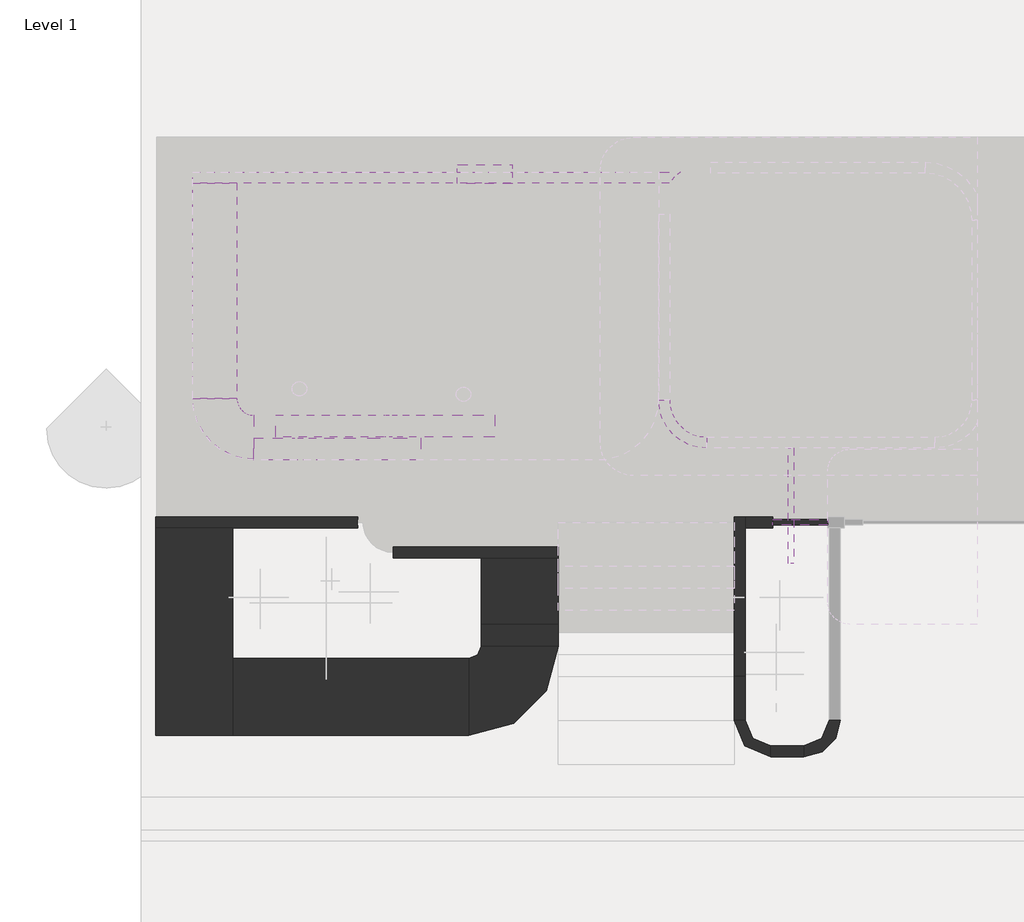
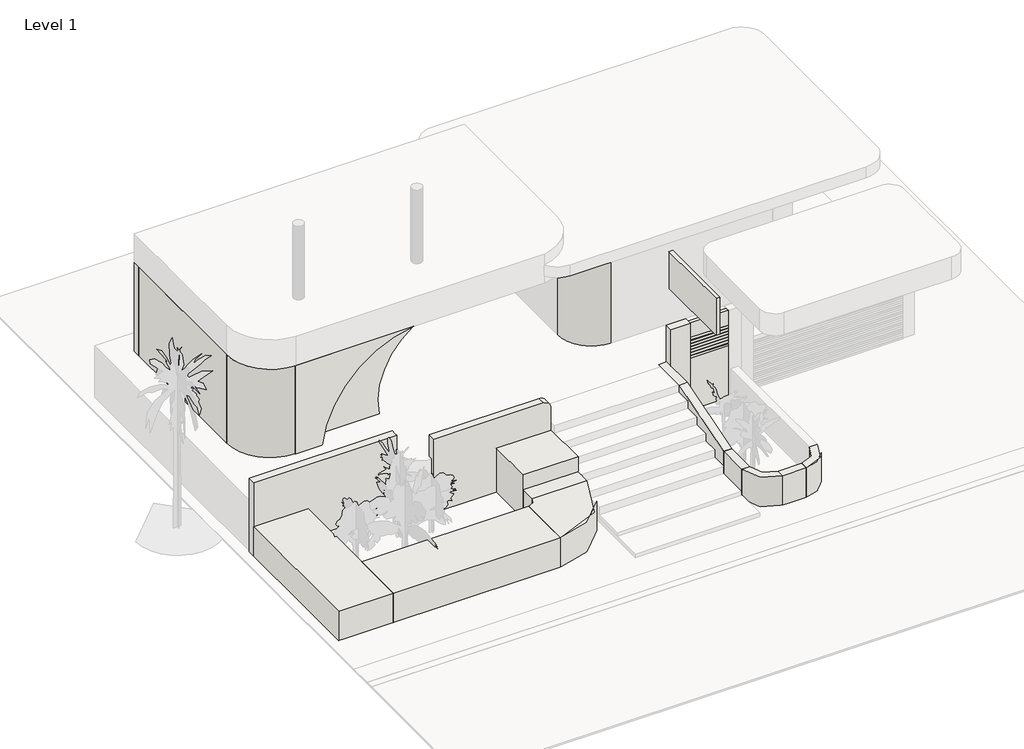
# One storey, part 1 of 2: 23 walls, 1 window.
"""IFC4 building model written with IfcOpenShell, lengths in millimetres."""

from ifc_helpers import new_model, si_unit, point, frame, frame_2d, origin, origin_with_axes, place, context, project, spatial, polyline, circle_curve, trimmed, segment, composite_curve, outline, extrude, faceted_brep, transform, mapped, element, save
from ifc_brep_helpers import plane_surface, cylinder_surface, revolved_surface, advanced_brep
from components import window_e9f06afb

model = new_model("IFC4")

# Units and contexts
model_context = context("Model", 3, world=origin())
ifc_project = project(units=[si_unit("LENGTHUNIT", "METRE", prefix="MILLI")], contexts=[model_context])

# Site, building, storey
site = spatial("IfcSite", under=ifc_project)
building = spatial("IfcBuilding", under=site)
storey = spatial("IfcBuildingStorey", under=building, Name="Level 1", Elevation=0.0)

# Walls
placement = place(None, origin())
element("IfcWall", 1, ObjectType="Generic - 12\" white", at=placement, inside=storey, context=model_context, shape_type="SweptSolid", body=[
    extrude(outline(composite_curve([segment(polyline([(0.0, -6972.7035766), (2743.2, -6972.7035766)]), True, "CONTINUOUS"), segment(trimmed(circle_curve(frame_2d((2743.2, -7277.5035766)), 304.8), [point((2743.2, -6972.7035766))], [point((3048.0, -7277.5035766))], False, "CARTESIAN"), True, "CONTINUOUS"), segment(polyline([(3048.0, -7277.5035766), (3048.0, -11546.5074836), (0.0, -11546.5074836), (0.0, -6972.7035766)]), True, "CONTINUOUS")], self_intersect=False)), frame((0.0, 4157.34911, 0.0), z_axis=(0.0, 1.0, 0.0), x_axis=(0.0, 0.0, 1.0)), (0.0, 0.0, 1.0), 304.8),
])
element("IfcWall", 2, ObjectType="Generic - 12\" white", at=placement, inside=storey, context=model_context, shape_type="AdvancedBrep", body=[
    advanced_brep(
    [(-12522.0257411, 5297.0999244, 0.0), (-18123.3035766, 5297.0999244, 0.0), (-18123.3035766, 5297.0999244, 3048.0), (-12522.0257411, 5297.0999244, 3048.0), (-12522.0257411, 4992.2999244, 0.0), (-12522.0257411, 4992.2999244, 3048.0), (-18123.3035766, 4992.2999244, 3048.0), (-18123.3035766, 4992.2999244, 1219.2), (-18123.3035766, 4992.2999244, 0.0), (-15989.7035766, 4992.2999244, 0.0)],
    [
        (0, 1),
        (1, 2),
        (2, 3),
        (3, 0),
        (4, 5),
        (5, 6),
        (6, 7),
        (7, 8),
        (8, 9),
        (9, 4),
        (0, 4, circle_curve(frame((-11546.5074836, 5144.6999244, 0.0), z_axis=(0.0, 0.0, 1.0), x_axis=(1.0, 0.0, 0.0)), 987.3508144)),
        (8, 1),
        (2, 6),
        (5, 3, circle_curve(frame((-11546.5074836, 5144.6999244, 3048.0), z_axis=(0.0, 0.0, -1.0), x_axis=(1.0, 0.0, 0.0)), 987.3508144)),
    ],
    [
        plane_surface(frame((-11670.258298, 5297.0999244, 0.0), z_axis=(0.0, 1.0, 0.0), x_axis=(-1.0, 0.0, 0.0))),
        plane_surface(frame((-11670.258298, 4992.2999244, 0.0), z_axis=(0.0, -1.0, 0.0), x_axis=(1.0, 0.0, 0.0))),
        plane_surface(frame((-12381.458298, 5297.0999244, 0.0), z_axis=(0.0, 0.0, -1.0), x_axis=(0.0, -1.0, 0.0))),
        plane_surface(frame((-17056.5035766, 5297.0999244, 3048.0), z_axis=(0.0, 0.0, 1.0), x_axis=(0.0, -1.0, 0.0))),
        revolved_surface(polyline([(-10559.1566692, 5144.6999244, 3048.0), (-10559.1566692, 5144.6999244, 0.0)]), (-11546.5074836, 5144.6999244, 0.0), (0.0, 0.0, 1.0)),
        plane_surface(frame((-18123.3035766, 4992.2999244, 0.0), z_axis=(-1.0, 0.0, 0.0), x_axis=(0.0, -1.0, 0.0))),
    ],
    [
        (0, [[1, 2, 3, 4]]),
        (1, [[5, 6, 7, 8, 9, 10]]),
        (2, [[-1, 11, -10, -9, 12]]),
        (3, [[-3, 13, -6, 14]]),
        (4, [[-4, -14, -5, -11]]),
        (5, [[-2, -12, -8, -7, -13]]),
    ],
),
])
element("IfcWall", 3, ObjectType="Generic - 12\" white", at=placement, inside=storey, context=model_context, shape_type="Brep", body=[
    faceted_brep([(-2095.9035766, 5297.0999244, 0.0), (-2095.9035766, 877.4999244, 0.0), (-2095.9035766, 877.4999244, 1219.2), (-2095.9035766, 3900.0999244, 2133.6), (-2095.9035766, 5297.0999244, 2133.6), (-1791.1035766, 5297.0999244, 0.0), (-1791.1035766, 5297.0999244, 2133.6), (-1791.1035766, 3900.0999244, 2133.6), (-1791.1035766, 877.4999244, 1219.2), (-1791.1035766, 877.4999244, 0.0), (-1791.1035766, 4992.2999244, 0.0)], [[[0, 1, 2, 3, 4]], [[5, 6, 7, 8, 9, 10]], [[1, 0, 5, 10, 9]], [[2, 1, 9, 8]], [[4, 3, 7, 6]], [[3, 2, 8, 7]], [[0, 4, 6, 5]]]),
])
element("IfcWall", 4, ObjectType="Generic - 12\" white", at=placement, inside=storey, context=model_context, shape_type="SweptSolid", body=[
    extrude(outline(polyline([(-2095.9035766, -341.7000756), (-2095.9035766, 877.4999244), (-1791.1035766, 877.4999244), (-1791.1035766, -341.7000756), (-2095.9035766, -341.7000756)])), origin_with_axes(), (0.0, 0.0, 1.0), 1219.2),
])
element("IfcWall", 5, ObjectType="Generic - 12\" white", at=placement, inside=storey, context=model_context, shape_type="SweptSolid", body=[
    extrude(outline(composite_curve([segment(polyline([(-1081.398989, -1051.4046632), (-1081.398989, -1356.2046632)]), True, "CONTINUOUS"), segment(trimmed(circle_curve(frame_2d((-1081.398989, -341.7000756)), 1014.5045876), [point((-1081.398989, -1356.2046632))], [point((-2095.9035766, -341.7000756))], False, "CARTESIAN"), True, "CONTINUOUS"), segment(polyline([(-2095.9035766, -341.7000756), (-1791.1035766, -341.7000756)]), True, "CONTINUOUS"), segment(trimmed(circle_curve(frame_2d((-1081.398989, -341.7000756)), 709.7045876), [point((-1791.1035766, -341.7000756))], [point((-1081.398989, -1051.4046632))], True, "CARTESIAN"), True, "CONTINUOUS")], self_intersect=False)), origin_with_axes(), (0.0, 0.0, 1.0), 1219.2),
])
element("IfcWall", 6, ObjectType="Generic - 12\" white", at=placement, inside=storey, context=model_context, shape_type="SweptSolid", body=[
    extrude(outline(polyline([(-166.998989, -1356.2046632), (-1081.398989, -1356.2046632), (-1081.398989, -1051.4046632), (-166.998989, -1051.4046632), (-166.998989, -1356.2046632)])), origin_with_axes(), (0.0, 0.0, 1.0), 1219.2),
])
element("IfcWall", 7, ObjectType="Generic - 12\" white", at=placement, inside=storey, context=model_context, shape_type="SweptSolid", body=[
    extrude(outline(composite_curve([segment(polyline([(542.7055987, -341.7000756), (847.5055987, -341.7000756)]), True, "CONTINUOUS"), segment(trimmed(circle_curve(frame_2d((-166.998989, -341.7000756)), 1014.5045876), [point((847.5055987, -341.7000756))], [point((-166.998989, -1356.2046632))], False, "CARTESIAN"), True, "CONTINUOUS"), segment(polyline([(-166.998989, -1356.2046632), (-166.998989, -1051.4046632)]), True, "CONTINUOUS"), segment(trimmed(circle_curve(frame_2d((-166.998989, -341.7000756)), 709.7045876), [point((-166.998989, -1051.4046632))], [point((542.7055987, -341.7000756))], True, "CARTESIAN"), True, "CONTINUOUS")], self_intersect=False)), origin_with_axes(), (0.0, 0.0, 1.0), 1219.2),
])
element("IfcWall", 8, ObjectType="Generic - 12\" white", at=placement, inside=storey, context=model_context, shape_type="Brep", body=[
    faceted_brep([(-1791.1035766, 4992.2999244, 0.0), (-1029.1035766, 4992.2999244, 0.0), (-1029.1035766, 4992.2999244, 3657.6), (-1791.1035766, 4992.2999244, 3657.6), (-1791.1035766, 5297.0999244, 0.0), (-1791.1035766, 5297.0999244, 2133.6), (-1791.1035766, 5297.0999244, 3657.6), (-1029.1035766, 5297.0999244, 3657.6), (-1029.1035766, 5297.0999244, 0.0), (-1029.1035766, 5220.8999244, 0.0), (-1029.1035766, 5068.4999244, 0.0)], [[[0, 1, 2, 3]], [[4, 5, 6, 7, 8]], [[1, 0, 4, 8, 9, 10]], [[3, 2, 7, 6]], [[0, 3, 6, 5, 4]], [[1, 10, 9, 8, 7, 2]]]),
])
element("IfcWall", 9, ObjectType="Generic - 12\" white", at=placement, inside=storey, context=model_context, shape_type="AdvancedBrep", body=[
    advanced_brep(
    [(-2854.0500691, 7504.6568058, 6096.0), (-3887.0438771, 8537.6506138, 6096.0), (-4191.8438771, 8537.6506138, 6096.0), (-2854.0500691, 7199.8568058, 6096.0), (-2854.0500691, 7504.6568058, 2133.6), (-2854.0500691, 7199.8568058, 2133.6), (-4191.8438771, 8537.6506138, 2133.6), (-3887.0438771, 8537.6506138, 2133.6), (-3887.0438771, 8537.6506138, 5791.2), (-4191.8438771, 8537.6506138, 5791.2)],
    [
        (0, 1, circle_curve(frame((-2854.0500691, 8537.6506138, 6096.0), z_axis=(0.0, 0.0, -1.0), x_axis=(1.0, 0.0, 0.0)), 1032.993808)),
        (1, 2),
        (2, 3, circle_curve(frame((-2854.0500691, 8537.6506138, 6096.0), z_axis=(0.0, 0.0, 1.0), x_axis=(1.0, 0.0, 0.0)), 1337.793808)),
        (3, 0),
        (4, 5),
        (5, 6, circle_curve(frame((-2854.0500691, 8537.6506138, 2133.6), z_axis=(0.0, 0.0, -1.0), x_axis=(1.0, 0.0, 0.0)), 1337.793808)),
        (6, 7),
        (7, 4, circle_curve(frame((-2854.0500691, 8537.6506138, 2133.6), z_axis=(0.0, 0.0, 1.0), x_axis=(1.0, 0.0, 0.0)), 1032.993808)),
        (0, 4),
        (7, 8),
        (8, 1),
        (6, 9),
        (9, 2),
        (5, 3),
    ],
    [
        plane_surface(frame((-1821.0562611, 8537.6506138, 6096.0), z_axis=(0.0, 0.0, 1.0), x_axis=(0.0, -1.0, 0.0))),
        plane_surface(frame((-1821.0562611, 8537.6506138, 2133.6), z_axis=(0.0, 0.0, -1.0), x_axis=(0.0, 1.0, 0.0))),
        revolved_surface(polyline([(-1821.0562611000003, 8537.6506138, 2133.6), (-1821.0562611000003, 8537.6506138, 6096.0)]), (-2854.0500691, 8537.6506138, 2133.6), (0.0, 0.0, -1.0)),
        plane_surface(frame((-3887.0438771, 8537.6506138, 6096.0), z_axis=(0.0, 1.0, 0.0), x_axis=(0.0, 0.0, -1.0))),
        cylinder_surface(frame((-2854.0500691, 8537.6506138, 2133.6), z_axis=(0.0, 0.0, 1.0), x_axis=(1.0, 0.0, 0.0)), 1337.793808),
        plane_surface(frame((-2854.0500691, 7199.8568058, 6096.0), z_axis=(1.0, 0.0, 0.0), x_axis=(0.0, 0.0, -1.0))),
    ],
    [
        (0, [[1, 2, 3, 4]]),
        (1, [[5, 6, 7, 8]]),
        (2, [[-1, 9, -8, 10, 11]]),
        (3, [[-2, -11, -10, -7, 12, 13]]),
        (4, [[-3, -13, -12, -6, 14]]),
        (5, [[-4, -14, -5, -9]]),
    ],
),
])
element("IfcWall", 10, ObjectType="Generic - 12\" white", at=placement, inside=storey, context=model_context, shape_type="AdvancedBrep", body=[
    advanced_brep(
    [(-3588.9235033, 14853.6629979, 2133.6), (-17097.1000691, 14853.6629979, 2133.6), (-17097.1000691, 14853.6629979, 5791.2), (-3588.9235033, 14853.6629979, 5791.2), (-5792.0438771, 14853.6629979, 2193.4133489), (-4191.8438771, 14853.6629979, 2193.4133489), (-4191.8438771, 14853.6629979, 5393.8133489), (-5792.0438771, 14853.6629979, 5393.8133489), (-9774.0964397, 14853.6629979, 2997.2), (-6738.7964397, 14853.6629979, 2997.2), (-6738.7964397, 14853.6629979, 5435.6), (-9774.0964397, 14853.6629979, 5435.6), (-17097.1000691, 14548.8629979, 2133.6), (-15877.9000691, 14548.8629979, 2133.6), (-3900.9068004, 14548.8629979, 2133.6), (-3900.9068004, 14548.8629979, 5791.2), (-15877.9000691, 14548.8629979, 5791.2), (-17097.1000691, 14548.8629979, 5791.2), (-4191.8438771, 14548.8629979, 2193.4133489), (-5792.0438771, 14548.8629979, 2193.4133489), (-5792.0438771, 14548.8629979, 5393.8133489), (-4191.8438771, 14548.8629979, 5393.8133489), (-9774.0964397, 14548.8629979, 5435.6), (-6738.7964397, 14548.8629979, 5435.6), (-6738.7964397, 14548.8629979, 2997.2), (-9774.0964397, 14548.8629979, 2997.2)],
    [
        (0, 1),
        (1, 2),
        (2, 3),
        (3, 0),
        (4, 5),
        (5, 6),
        (6, 7),
        (7, 4),
        (8, 9),
        (9, 10),
        (10, 11),
        (11, 8),
        (12, 13),
        (13, 14),
        (14, 15),
        (15, 16),
        (16, 17),
        (17, 12),
        (18, 19),
        (19, 20),
        (20, 21),
        (21, 18),
        (22, 23),
        (23, 24),
        (24, 25),
        (25, 22),
        (3, 15, circle_curve(frame((-2746.2869957, 13679.0999244, 5791.2), z_axis=(0.0, 0.0, 1.0), x_axis=(1.0, 0.0, 0.0)), 1445.5568814)),
        (14, 0, circle_curve(frame((-2746.2869957, 13679.0999244, 2133.6), z_axis=(0.0, 0.0, -1.0), x_axis=(1.0, 0.0, 0.0)), 1445.5568814)),
        (12, 1),
        (2, 17),
        (4, 19),
        (18, 5),
        (21, 6),
        (20, 7),
        (24, 9),
        (8, 25),
        (23, 10),
        (22, 11),
    ],
    [
        plane_surface(frame((-3538.3964397, 14853.6629979, 2133.6), z_axis=(0.0, 1.0, 0.0), x_axis=(-1.0, 0.0, 0.0))),
        plane_surface(frame((-3538.3964397, 14548.8629979, 2133.6), z_axis=(0.0, -1.0, 0.0), x_axis=(1.0, 0.0, 0.0))),
        revolved_surface(polyline([(-1300.7301142999997, 13679.0999244, 5791.2), (-1300.7301142999997, 13679.0999244, 2133.6)]), (-2746.2869957, 13679.0999244, 2133.6), (0.0, 0.0, 1.0)),
        plane_surface(frame((-3538.3964397, 14853.6629979, 2133.6), z_axis=(0.0, 0.0, -1.0), x_axis=(0.0, -1.0, 0.0))),
        plane_surface(frame((-16487.5000691, 14853.6629979, 5791.2), z_axis=(0.0, 0.0, 1.0), x_axis=(0.0, -1.0, 0.0))),
        plane_surface(frame((-5792.0438771, 14853.6629979, 2193.4133489), z_axis=(0.0, 0.0, 1.0), x_axis=(0.0, -1.0, 0.0))),
        plane_surface(frame((-4191.8438771, 14853.6629979, 2193.4133489), z_axis=(-1.0, 0.0, 0.0), x_axis=(0.0, -1.0, 0.0))),
        plane_surface(frame((-4191.8438771, 14853.6629979, 5393.8133489), z_axis=(0.0, 0.0, -1.0), x_axis=(0.0, -1.0, 0.0))),
        plane_surface(frame((-5792.0438771, 14853.6629979, 5393.8133489), z_axis=(1.0, 0.0, 0.0), x_axis=(0.0, -1.0, 0.0))),
        plane_surface(frame((-8262.7964397, 13329.6629979, 2997.2), z_axis=(0.0, 0.0, 1.0), x_axis=(0.0, 1.0, 0.0))),
        plane_surface(frame((-6738.7964397, 13329.6629979, 2997.2), z_axis=(-1.0, 0.0, 0.0), x_axis=(0.0, 1.0, 0.0))),
        plane_surface(frame((-6738.7964397, 13329.6629979, 5435.6), z_axis=(0.0, 0.0, -1.0), x_axis=(0.0, 1.0, 0.0))),
        plane_surface(frame((-9774.0964397, 13329.6629979, 5435.6), z_axis=(1.0, 0.0, 0.0), x_axis=(0.0, 1.0, 0.0))),
        plane_surface(frame((-17097.1000691, 14701.2629979, 2133.6), z_axis=(-1.0, 0.0, 0.0), x_axis=(0.0, -1.0, 0.0))),
    ],
    [
        (0, [[1, 2, 3, 4], [5, 6, 7, 8], [9, 10, 11, 12]]),
        (1, [[13, 14, 15, 16, 17, 18], [19, 20, 21, 22], [23, 24, 25, 26]]),
        (2, [[-4, 27, -15, 28]]),
        (3, [[-1, -28, -14, -13, 29]]),
        (4, [[-3, 30, -17, -16, -27]]),
        (5, [[-5, 31, -19, 32]]),
        (6, [[-6, -32, -22, 33]]),
        (7, [[-7, -33, -21, 34]]),
        (8, [[-8, -34, -20, -31]]),
        (9, [[35, -9, 36, -25]]),
        (10, [[37, -10, -35, -24]]),
        (11, [[-37, -23, 38, -11]]),
        (12, [[-38, -26, -36, -12]]),
        (13, [[-2, -29, -18, -30]]),
    ],
),
])
element("IfcWall", 11, ObjectType="Generic - 2'", at=placement, inside=storey, context=model_context, shape_type="AdvancedBrep", body=[
    advanced_brep(
    [(-14800.2693346, 7502.2322633, 5791.2), (-14800.2693346, 7502.2322633, 2133.6), (-11752.2693346, 7502.2322633, 2133.6), (-8736.0193346, 7502.2322633, 5791.2), (-14800.2693346, 8111.8322633, 5791.2), (-8736.0193346, 8111.8322633, 5791.2), (-11752.2693346, 8111.8322633, 2133.6), (-14800.2693346, 8111.8322633, 2133.6)],
    [
        (0, 1),
        (1, 2),
        (2, 3, circle_curve(frame((-8736.0193346, 7502.2322633, 2718.7205295), z_axis=(0.0, 1.0, 0.0), x_axis=(-1.0, 0.0, 0.0)), 3072.4794705)),
        (3, 0),
        (4, 5),
        (5, 6, circle_curve(frame((-8736.0193346, 8111.8322633, 2718.7205295), z_axis=(0.0, -1.0, 0.0), x_axis=(-1.0, 0.0, 0.0)), 3072.4794705)),
        (6, 7),
        (7, 4),
        (1, 7),
        (6, 2),
        (3, 5),
        (4, 0),
    ],
    [
        plane_surface(frame((-14800.2693346, 7502.2322633, 5791.2), z_axis=(0.0, -1.0, 0.0), x_axis=(0.0, 0.0, -1.0))),
        plane_surface(frame((-14800.2693346, 8111.8322633, 5791.2), z_axis=(0.0, 1.0, 0.0), x_axis=(0.0, 0.0, 1.0))),
        plane_surface(frame((-14800.2693346, 7502.2322633, 2133.6), z_axis=(0.0, 0.0, -1.0), x_axis=(0.0, 1.0, 0.0))),
        plane_surface(frame((-8736.0193346, 7502.2322633, 5791.2), z_axis=(0.0, 0.0, 1.0), x_axis=(0.0, 1.0, 0.0))),
        plane_surface(frame((-14800.2693346, 7502.2322633, 5791.2), z_axis=(-1.0, 0.0, 0.0), x_axis=(0.0, 1.0, 0.0))),
        revolved_surface(polyline([(-11808.4988051, 8111.8322633, 2718.7205295), (-11808.4988051, 7502.2322633, 2718.7205295)]), (-8736.0193346, 8111.8322633, 2718.7205295), (0.0, 1.0, 0.0)),
    ],
    [
        (0, [[1, 2, 3, 4]]),
        (1, [[5, 6, 7, 8]]),
        (2, [[-2, 9, -7, 10]]),
        (3, [[-4, 11, -5, 12]]),
        (4, [[-1, -12, -8, -9]]),
        (5, [[-3, -10, -6, -11]]),
    ],
),
])
element("IfcWall", 12, ObjectType="Generic - 2'", at=placement, inside=storey, context=model_context, shape_type="AdvancedBrep", body=[
    advanced_brep(
    [(-15409.8693346, 6873.8139644, 2133.6), (-14343.0693346, 6873.8139644, 2133.6), (-10776.892063, 6873.8139644, 5791.2), (-15409.8693346, 6873.8139644, 5791.2), (-15409.8693346, 7483.4139644, 2133.6), (-15409.8693346, 7483.4139644, 5791.2), (-10776.892063, 7483.4139644, 5791.2), (-14343.0693346, 7483.4139644, 2133.6), (-15409.8693346, 6892.6322633, 2133.6), (-15409.8693346, 6892.6322633, 5791.2)],
    [
        (0, 1),
        (1, 2, circle_curve(frame((-10246.3978198, 6873.8139644, 1706.6457679), z_axis=(0.0, 1.0, 0.0), x_axis=(-1.0, 0.0, 0.0)), 4118.8599657)),
        (2, 3),
        (3, 0),
        (4, 5),
        (5, 6),
        (6, 7, circle_curve(frame((-10246.3978198, 7483.4139644, 1706.6457679), z_axis=(0.0, -1.0, 0.0), x_axis=(-1.0, 0.0, 0.0)), 4118.8599657)),
        (7, 4),
        (0, 8),
        (8, 4),
        (7, 1),
        (2, 6),
        (5, 9),
        (9, 3),
    ],
    [
        plane_surface(frame((-15409.8693346, 6873.8139644, 2133.6), z_axis=(0.0, -1.0, 0.0), x_axis=(1.0, 0.0, 0.0))),
        plane_surface(frame((-15409.8693346, 7483.4139644, 2133.6), z_axis=(0.0, 1.0, 0.0), x_axis=(-1.0, 0.0, 0.0))),
        plane_surface(frame((-15409.8693346, 6873.8139644, 2133.6), z_axis=(0.0, 0.0, -1.0), x_axis=(0.0, 1.0, 0.0))),
        plane_surface(frame((-10776.892063, 6873.8139644, 5791.2), z_axis=(0.0, 0.0, 1.0), x_axis=(0.0, 1.0, 0.0))),
        plane_surface(frame((-15409.8693346, 6873.8139644, 5791.2), z_axis=(-1.0, 0.0, 0.0), x_axis=(0.0, 1.0, 0.0))),
        revolved_surface(polyline([(-14365.257785500002, 7483.4139644, 1706.6457679), (-14365.257785500002, 6873.8139644, 1706.6457679)]), (-10246.3978198, 7483.4139644, 1706.6457679), (0.0, 1.0, 0.0)),
    ],
    [
        (0, [[1, 2, 3, 4]]),
        (1, [[5, 6, 7, 8]]),
        (2, [[-1, 9, 10, -8, 11]]),
        (3, [[-3, 12, -6, 13, 14]]),
        (4, [[-4, -14, -13, -5, -10, -9]]),
        (5, [[-2, -11, -7, -12]]),
    ],
),
])
element("IfcWall", 13, ObjectType="Generic - 4' white", at=placement, inside=storey, context=model_context, shape_type="SweptSolid", body=[
    extrude(outline(polyline([(-17097.1000691, 8579.8629979), (-17097.1000691, 14548.8629979), (-15877.9000691, 14548.8629979), (-15877.9000691, 8579.8629979), (-17097.1000691, 8579.8629979)])), frame((0.0, 0.0, 2133.6), z_axis=(0.0, 0.0, 1.0), x_axis=(1.0, 0.0, 0.0)), (0.0, 0.0, 1.0), 3657.6),
])
element("IfcWall", 14, ObjectType="Generic - 4' white", at=placement, inside=storey, context=model_context, shape_type="AdvancedBrep", body=[
    advanced_brep(
    [(-15409.8693346, 8111.8322633, 5791.2), (-15877.9000691, 8579.8629979, 5791.2), (-17097.1000691, 8579.8629979, 5791.2), (-15409.8693346, 6892.6322633, 5791.2), (-15409.8693346, 7483.4139644, 5791.2), (-15409.8693346, 8111.8322633, 2133.6), (-15409.8693346, 7483.4139644, 2133.6), (-15409.8693346, 6892.6322633, 2133.6), (-17097.1000691, 8579.8629979, 2133.6), (-15877.9000691, 8579.8629979, 2133.6)],
    [
        (0, 1, circle_curve(frame((-15409.8693346, 8579.8629979, 5791.2), z_axis=(0.0, 0.0, -1.0), x_axis=(1.0, 0.0, 0.0)), 468.0307345)),
        (1, 2),
        (2, 3, circle_curve(frame((-15409.8693346, 8579.8629979, 5791.2), z_axis=(0.0, 0.0, 1.0), x_axis=(1.0, 0.0, 0.0)), 1687.2307345)),
        (3, 4),
        (4, 0),
        (5, 6),
        (6, 7),
        (7, 8, circle_curve(frame((-15409.8693346, 8579.8629979, 2133.6), z_axis=(0.0, 0.0, -1.0), x_axis=(1.0, 0.0, 0.0)), 1687.2307345)),
        (8, 9),
        (9, 5, circle_curve(frame((-15409.8693346, 8579.8629979, 2133.6), z_axis=(0.0, 0.0, 1.0), x_axis=(1.0, 0.0, 0.0)), 468.0307345)),
        (0, 5),
        (9, 1),
        (8, 2),
        (7, 3),
    ],
    [
        plane_surface(frame((-14941.8386001, 8579.8629979, 5791.2), z_axis=(0.0, 0.0, 1.0), x_axis=(0.0, -1.0, 0.0))),
        plane_surface(frame((-14941.8386001, 8579.8629979, 2133.6), z_axis=(0.0, 0.0, -1.0), x_axis=(0.0, 1.0, 0.0))),
        revolved_surface(polyline([(-14941.8386001, 8579.8629979, 2133.6), (-14941.8386001, 8579.8629979, 5791.2)]), (-15409.8693346, 8579.8629979, 2133.6), (0.0, 0.0, -1.0)),
        plane_surface(frame((-15877.9000691, 8579.8629979, 5791.2), z_axis=(0.0, 1.0, 0.0), x_axis=(0.0, 0.0, -1.0))),
        cylinder_surface(frame((-15409.8693346, 8579.8629979, 2133.6), z_axis=(0.0, 0.0, 1.0), x_axis=(1.0, 0.0, 0.0)), 1687.2307345),
        plane_surface(frame((-15409.8693346, 6892.6322633, 5791.2), z_axis=(1.0, 0.0, 0.0), x_axis=(0.0, 0.0, -1.0))),
    ],
    [
        (0, [[1, 2, 3, 4, 5]]),
        (1, [[6, 7, 8, 9, 10]]),
        (2, [[-1, 11, -10, 12]]),
        (3, [[-2, -12, -9, 13]]),
        (4, [[-3, -13, -8, 14]]),
        (5, [[-5, -4, -14, -7, -6, -11]]),
    ],
),
])
element("IfcWall", 15, ObjectType="Generic - 6\" brown", at=placement, inside=storey, context=model_context, shape_type="SweptSolid", body=[
    extrude(outline(polyline([(494.8964234, 5068.4999244), (-1029.1035766, 5068.4999244), (-1029.1035766, 5220.8999244), (494.8964234, 5220.8999244), (494.8964234, 5068.4999244)])), frame((0.0, 0.0, 2133.6), z_axis=(0.0, 0.0, 1.0), x_axis=(1.0, 0.0, 0.0)), (0.0, 0.0, 1.0), 101.6),
    extrude(outline(polyline([(494.8964234, 5068.4999244), (-1029.1035766, 5068.4999244), (-1029.1035766, 5220.8999244), (494.8964234, 5220.8999244), (494.8964234, 5068.4999244)])), frame((0.0, 0.0, 2260.6), z_axis=(0.0, 0.0, 1.0), x_axis=(1.0, 0.0, 0.0)), (0.0, 0.0, 1.0), 101.6),
    extrude(outline(polyline([(494.8964234, 5068.4999244), (-1029.1035766, 5068.4999244), (-1029.1035766, 5220.8999244), (494.8964234, 5220.8999244), (494.8964234, 5068.4999244)])), frame((0.0, 0.0, 2387.6), z_axis=(0.0, 0.0, 1.0), x_axis=(1.0, 0.0, 0.0)), (0.0, 0.0, 1.0), 101.6),
    extrude(outline(polyline([(494.8964234, 5068.4999244), (-1029.1035766, 5068.4999244), (-1029.1035766, 5220.8999244), (494.8964234, 5220.8999244), (494.8964234, 5068.4999244)])), frame((0.0, 0.0, 2514.6), z_axis=(0.0, 0.0, 1.0), x_axis=(1.0, 0.0, 0.0)), (0.0, 0.0, 1.0), 101.6),
    extrude(outline(polyline([(494.8964234, 5068.4999244), (-1029.1035766, 5068.4999244), (-1029.1035766, 5220.8999244), (494.8964234, 5220.8999244), (494.8964234, 5068.4999244)])), frame((0.0, 0.0, 2641.6), z_axis=(0.0, 0.0, 1.0), x_axis=(1.0, 0.0, 0.0)), (0.0, 0.0, 1.0), 101.6),
    extrude(outline(polyline([(494.8964234, 5068.4999244), (-1029.1035766, 5068.4999244), (-1029.1035766, 5220.8999244), (494.8964234, 5220.8999244), (494.8964234, 5068.4999244)])), frame((0.0, 0.0, 2768.6), z_axis=(0.0, 0.0, 1.0), x_axis=(1.0, 0.0, 0.0)), (0.0, 0.0, 1.0), 101.6),
    extrude(outline(polyline([(494.8964234, 5068.4999244), (-1029.1035766, 5068.4999244), (-1029.1035766, 5220.8999244), (494.8964234, 5220.8999244), (494.8964234, 5068.4999244)])), frame((0.0, 0.0, 2895.6), z_axis=(0.0, 0.0, 1.0), x_axis=(1.0, 0.0, 0.0)), (0.0, 0.0, 1.0), 101.6),
])
element("IfcWall", 16, ObjectType="Generic - 6\" white", at=placement, inside=storey, context=model_context, shape_type="SweptSolid", body=[
    extrude(outline(polyline([(494.8964234, 5068.4999244), (-1029.1035766, 5068.4999244), (-1029.1035766, 5220.8999244), (494.8964234, 5220.8999244), (494.8964234, 5068.4999244)])), origin_with_axes(), (0.0, 0.0, 1.0), 2133.6),
])
element("IfcWall", 17, ObjectType="Generic - 6\" white", at=placement, inside=storey, context=model_context, shape_type="SweptSolid", body=[
    extrude(outline(polyline([(494.8964234, 5068.4999244), (-1029.1035766, 5068.4999244), (-1029.1035766, 5220.8999244), (494.8964234, 5220.8999244), (494.8964234, 5068.4999244)])), frame((0.0, 0.0, 2997.2), z_axis=(0.0, 0.0, 1.0), x_axis=(1.0, 0.0, 0.0)), (0.0, 0.0, 1.0), 609.6),
])
element("IfcWall", 18, ObjectType="Generic - 6\" white", at=placement, inside=storey, context=model_context, shape_type="SweptSolid", body=[
    extrude(outline(polyline([(-600.2944013, 3999.4568058), (-600.2944013, 7199.8568058), (-447.8944013, 7199.8568058), (-447.8944013, 3999.4568058), (-600.2944013, 3999.4568058)])), frame((0.0, 0.0, 3606.8), z_axis=(0.0, 0.0, 1.0), x_axis=(1.0, 0.0, 0.0)), (0.0, 0.0, 1.0), 1524.0),
])
element("IfcWall", 19, ObjectType="Generic - 7' white 2", at=placement, inside=storey, context=model_context, shape_type="Brep", body=[
    faceted_brep([(-9106.3035766, 4146.8793884, 0.0), (-9106.3035766, 2318.0793884, 0.0), (-9106.3035766, 2318.0793884, 1219.2), (-9106.3035766, 2318.0793884, 1828.8), (-9106.3035766, 4146.8793884, 1828.8), (-6972.7035766, 4146.8793884, 0.0), (-6972.7035766, 4146.8793884, 1828.8), (-6972.7035766, 2318.0793884, 1828.8), (-6972.7035766, 2318.0793884, 1219.2), (-6972.7035766, 2318.0793884, 0.0)], [[[0, 1, 2, 3, 4]], [[5, 6, 7, 8, 9]], [[1, 0, 5, 9]], [[3, 2, 1, 9, 8, 7]], [[4, 3, 7, 6]], [[0, 4, 6, 5]]]),
])
element("IfcWall", 20, ObjectType="Generic - 7' white 2", at=placement, inside=storey, context=model_context, shape_type="SweptSolid", body=[
    extrude(outline(polyline([(-9106.3035766, 1708.4793884), (-9106.3035766, 2318.0793884), (-6972.7035766, 2318.0793884), (-6972.7035766, 1708.4793884), (-9106.3035766, 1708.4793884)])), origin_with_axes(), (0.0, 0.0, 1.0), 1219.2),
])
element("IfcWall", 21, ObjectType="Generic - 7' white 2", at=placement, inside=storey, context=model_context, shape_type="SweptSolid", body=[
    extrude(outline(composite_curve([segment(polyline([(-9447.314473, -766.131508), (-9447.314473, 1367.468492)]), True, "CONTINUOUS"), segment(trimmed(circle_curve(frame_2d((-9447.314473, 1708.4793884)), 341.0108964), [point((-9447.314473, 1367.468492))], [point((-9106.3035766, 1708.4793884))], True, "CARTESIAN"), True, "CONTINUOUS"), segment(polyline([(-9106.3035766, 1708.4793884), (-6972.7035766, 1708.4793884)]), True, "CONTINUOUS"), segment(trimmed(circle_curve(frame_2d((-9447.314473, 1708.4793884)), 2474.6108964), [point((-6972.7035766, 1708.4793884))], [point((-9447.314473, -766.131508))], False, "CARTESIAN"), True, "CONTINUOUS")], self_intersect=False)), origin_with_axes(), (0.0, 0.0, 1.0), 1219.2),
])
element("IfcWall", 22, ObjectType="Generic - 7' white 2", at=placement, inside=storey, context=model_context, shape_type="SweptSolid", body=[
    extrude(outline(polyline([(-15989.7035766, 1367.468492), (-9447.314473, 1367.468492), (-9447.314473, -766.131508), (-15989.7035766, -766.131508), (-15989.7035766, 1367.468492)])), origin_with_axes(), (0.0, 0.0, 1.0), 1219.2),
])
element("IfcWall", 23, ObjectType="Generic - 7' white 2", at=placement, inside=storey, context=model_context, shape_type="Brep", body=[
    faceted_brep([(-18123.3035766, 4992.2999244, 0.0), (-18123.3035766, -766.131508, 0.0), (-18123.3035766, -766.131508, 1219.2), (-18123.3035766, 4992.2999244, 1219.2), (-15989.7035766, 4992.2999244, 0.0), (-15989.7035766, 4992.2999244, 1219.2), (-15989.7035766, 1367.468492, 1219.2), (-15989.7035766, -766.131508, 1219.2), (-15989.7035766, -766.131508, 0.0), (-15989.7035766, 1367.468492, 0.0)], [[[0, 1, 2, 3]], [[4, 5, 6, 7, 8, 9]], [[1, 0, 4, 9, 8]], [[3, 2, 7, 6, 5]], [[2, 1, 8, 7]], [[0, 3, 5, 4]]]),
])

# Window
window_shape = window_e9f06afb(model_context)
element("IfcWindow", 24, ObjectType="Instance - Fixed.0001 : 60\" x 96\"", at=placement, inside=storey, context=model_context, shape_type="MappedRepresentation", body=[
    mapped(window_shape, transform((-9050.1964397, 14701.2629979, 2387.6), x_axis=(-1.0, 0.0, 0.0), y_axis=(0.0, -1.0, 0.0), z_axis=(0.0, 0.0, 1.0))),
])

save(model, "model.ifc")

# Revit data of these elements
# Type "Generic - 12\" white"
#   Assembly Code = "B2010"
#   Layers, outside or top first: 1' - 0" "Door - Frame" (function 1)
# Type "Generic - 2'"
#   Assembly Code = "B2010"
#   Layers, outside or top first: 2' - 0" "Door - Frame" (function 1)
# Type "Generic - 4' white"
#   Assembly Code = "B2010"
#   Layers, outside or top first: 4' - 0" "Door - Frame" (function 1)
# Type "Generic - 6\" brown"
#   Assembly Code = "B2010"
#   Layers, outside or top first: 0' - 6" "Door - Panel" (function 1)
# Type "Generic - 6\" white"
#   Assembly Code = "B2010"
#   Layers, outside or top first: 0' - 6" "Door - Frame" (function 1)
# Type "Generic - 7' white 2"
#   Assembly Code = "B2010"
#   Layers, outside or top first: 7' - 0" "Door - Frame" (function 1)
# Type "Instance - Fixed.0001 : 60\" x 96\""
#   Type Mark = "13"
#   Construction Type Id = "MDOOR"
#   Assembly Code = "B2020100"
#   Analytic Construction = "Metal"
#   Heat Transfer Coefficient (U) = 0.651978 BTU/(h·ft²·°F)
#   Height [instance default] = 6' - 0"
#   Default Sill Height = 2' - 0"
#   Width [instance default] = 3' - 0"
#   Window Inset = 1' - 6"
#   Define Thermal Properties by = 1
#   Glass Pane Material = Glass
#   Sash Material = Door - Frame
#   Visual Light Transmittance = 0
#   Thermal Resistance (R) = 0
#   Solar Heat Gain Coefficient = 0
#   Wall Closure = (empty or 0)
# Elements 1, 2 (IfcWall, "Generic - 12\" white")
#   Top Offset = 0' - 0"
#   Base Offset = 0' - 0"
#   Unconnected Height = 10' - 0"
#   wall height = 10' - 0"
#   Phase Created = New Construction
#   Base Constraint = Level 1
#   Materials on its faces: "Door - Frame"
# Element 3 (IfcWall, "Generic - 12\" white")
#   Top Offset = 0' - 0"
#   Base Offset = 0' - 0"
#   Unconnected Height = 7' - 0"
#   wall height = 7' - 0"
#   Phase Created = New Construction
#   Base Constraint = Level 1
#   Materials on its faces: "Door - Frame"
# Elements 4, 6 (IfcWall, "Generic - 12\" white")
#   Top Offset = 0' - 0"
#   Base Offset = 0' - 0"
#   Unconnected Height = 4' - 0"
#   wall height = 4' - 0"
#   Phase Created = New Construction
#   Base Constraint = Level 1
#   Materials on its faces: "Door - Frame"
# Elements 5, 7 (IfcWall, "Generic - 12\" white")
#   Top Offset = 0' - 0"
#   Base Offset = 0' - 0"
#   Unconnected Height = 4' - 0"
#   wall height = 4' - 0"
#   Phase Created = New Construction
#   Materials on its faces: "Door - Frame"
# Element 8 (IfcWall, "Generic - 12\" white")
#   Top Offset = 0' - 0"
#   Base Offset = 0' - 0"
#   Unconnected Height = 12' - 0"
#   wall height = 12' - 0"
#   Phase Created = New Construction
#   Base Constraint = Level 1
#   Materials on its faces: "Door - Frame"
# Element 9 (IfcWall, "Generic - 12\" white")
#   built-in parameter 1001111 = 7' - 0"
#   Top Offset = 0' - 0"
#   Base Offset = 7' - 0"
#   Unconnected Height = 13' - 0"
#   wall height = 13' - 0"
#   Phase Created = New Construction
#   Materials on its faces: "Door - Frame"
# Element 10 (IfcWall, "Generic - 12\" white")
#   built-in parameter 1001111 = 7' - 0"
#   Top Offset = 0' - 0"
#   Base Offset = 7' - 0"
#   Unconnected Height = 12' - 0"
#   wall height = 12' - 0"
#   Phase Created = New Construction
#   Base Constraint = Level 1
#   Materials on its faces: "Door - Frame"
# Elements 11, 12 (IfcWall, "Generic - 2'")
#   built-in parameter 1001111 = 7' - 0"
#   Top Offset = 0' - 0"
#   Base Offset = 7' - 0"
#   Unconnected Height = 12' - 0"
#   wall height = 12' - 0"
#   Phase Created = New Construction
#   Base Constraint = Level 1
#   Materials on its faces: "Door - Frame"
# Element 13 (IfcWall, "Generic - 4' white")
#   built-in parameter 1001111 = 7' - 0"
#   Top Offset = 0' - 0"
#   Base Offset = 7' - 0"
#   Unconnected Height = 12' - 0"
#   wall height = 12' - 0"
#   Phase Created = New Construction
#   Base Constraint = Level 1
#   Materials on its faces: "Door - Frame"
# Element 14 (IfcWall, "Generic - 4' white")
#   built-in parameter 1001111 = 7' - 0"
#   Top Offset = 0' - 0"
#   Base Offset = 7' - 0"
#   Unconnected Height = 12' - 0"
#   wall height = 12' - 0"
#   Phase Created = New Construction
#   Materials on its faces: "Door - Frame"
# Element 15 (IfcWall, "Generic - 6\" brown")
#   built-in parameter 1001111 = 7' - 0"
#   Top Offset = 0' - 0"
#   Base Offset = 7' - 0"
#   Unconnected Height = 3' - 0"
#   wall height = 3' - 0"
#   Phase Created = New Construction
#   Base Constraint = Level 1
#   Materials on its faces: "Door - Panel"
# Element 16 (IfcWall, "Generic - 6\" white")
#   Top Offset = 0' - 0"
#   Base Offset = 0' - 0"
#   Unconnected Height = 7' - 0"
#   wall height = 7' - 0"
#   Phase Created = New Construction
#   Base Constraint = Level 1
#   Materials on its faces: "Door - Frame"
# Element 17 (IfcWall, "Generic - 6\" white")
#   built-in parameter 1001111 = 9' - 10"
#   Top Offset = 0' - 0"
#   Base Offset = 9' - 10"
#   Unconnected Height = 2' - 0"
#   wall height = 2' - 0"
#   Phase Created = New Construction
#   Base Constraint = Level 1
#   Materials on its faces: "Door - Frame"
# Element 18 (IfcWall, "Generic - 6\" white")
#   built-in parameter 1001111 = 11' - 10"
#   Top Offset = 0' - 0"
#   Base Offset = 11' - 10"
#   Unconnected Height = 5' - 0"
#   wall height = 5' - 0"
#   Phase Created = New Construction
#   Base Constraint = Level 1
#   Materials on its faces: "Door - Frame"
# Element 19 (IfcWall, "Generic - 7' white 2")
#   Top Offset = 0' - 0"
#   Base Offset = 0' - 0"
#   Unconnected Height = 6' - 0"
#   wall height = 6' - 0"
#   Phase Created = New Construction
#   Base Constraint = Level 1
#   Materials on its faces: "Door - Frame"
# Elements 20, 22, 23 (IfcWall, "Generic - 7' white 2")
#   Top Offset = 0' - 0"
#   Base Offset = 0' - 0"
#   Unconnected Height = 4' - 0"
#   wall height = 4' - 0"
#   Phase Created = New Construction
#   Base Constraint = Level 1
#   Materials on its faces: "Door - Frame"
# Element 21 (IfcWall, "Generic - 7' white 2")
#   Top Offset = 0' - 0"
#   Base Offset = 0' - 0"
#   Unconnected Height = 4' - 0"
#   wall height = 4' - 0"
#   Phase Created = New Construction
#   Materials on its faces: "Door - Frame"
# Element 24 (IfcWindow, "Instance - Fixed.0001 : 60\" x 96\"")
#   Mark = "2"
#   Width = 5' - 0"
#   Height = 8' - 0"
#   Phase Created = New Construction
#   Materials on its faces: "Door - Frame", "Glass"
# Materials
#   "Door - Frame": colour RGB 118 70 51, transparency 0, Cost = 0
#   "Door - Panel": class "Wood", colour RGB 210 159 95, transparency 0, Cost = 0
#   "Glass": class "Glass", colour RGB 0 128 192, transparency 0.75, Description = "Soda Lime Glass", Cost = 0
